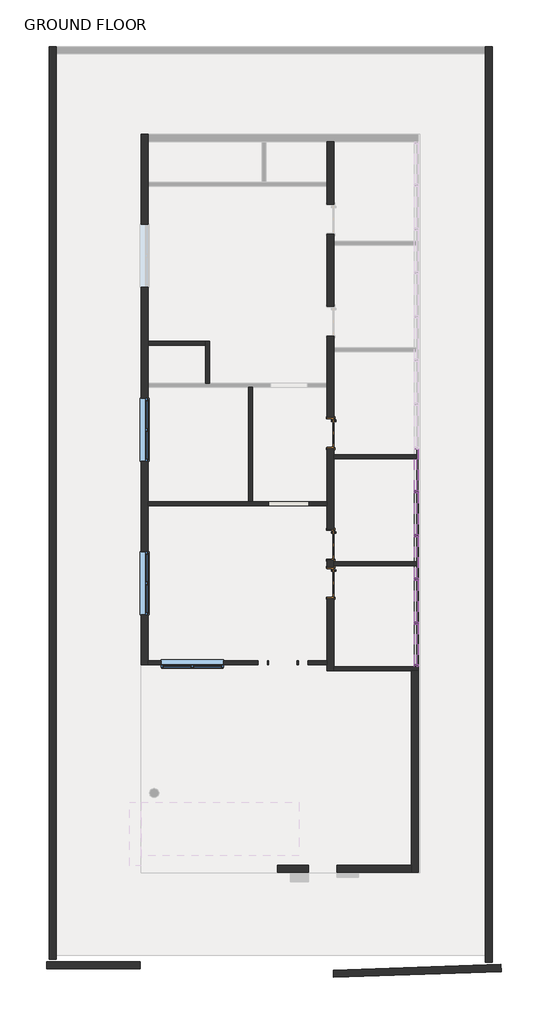
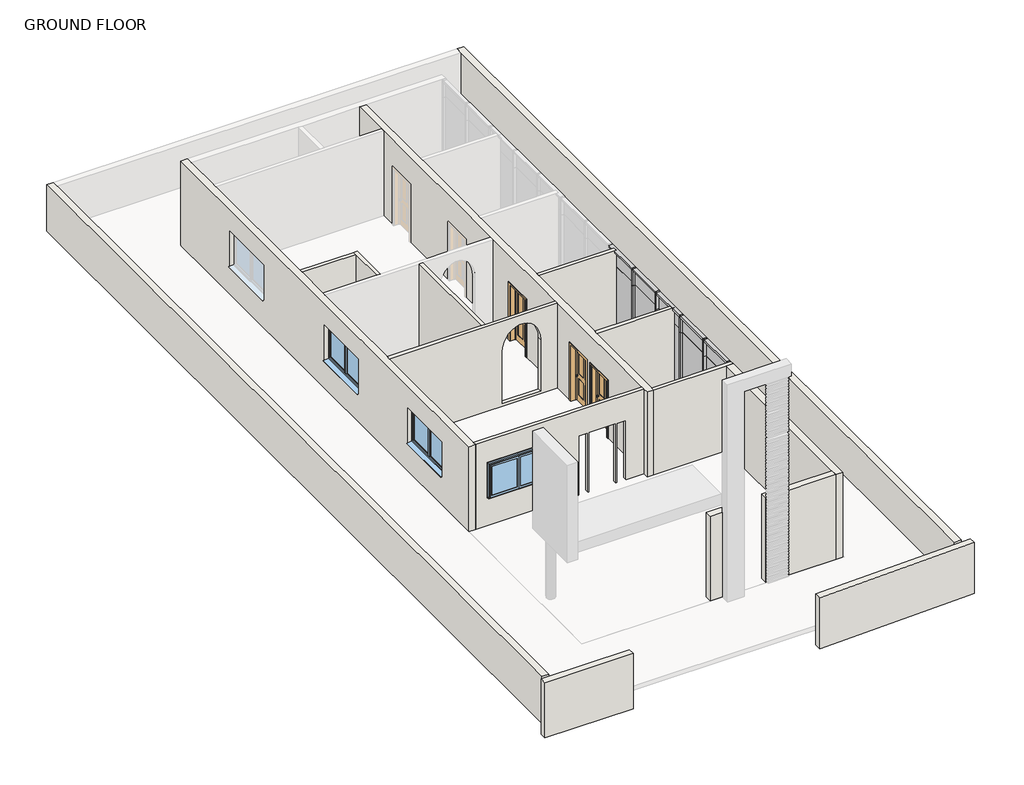
# One storey, part 1 of 2: 19 members, 16 walls, 10 plates, 3 doors, 3 windows.
"""IFC4 building model written with IfcOpenShell, lengths in millimetres."""

from ifc_helpers import new_model, si_unit, point, frame, origin, origin_with_axes, place, context, project, spatial, polyline, ellipse_curve, trimmed, outline, extrude, faceted_brep, transform, mapped, element, save
from ifc_brep_helpers import plane_surface, extruded_surface, advanced_brep
from components import door_8a5afc22, member_fe35c162, member_c919ac1a, member_ee409385, member_47bfaf8a, member_f0fea5a5, member_6e77e263, system_panel_glazed_23a28a9f, system_panel_glazed_17e06366, system_panel_glazed_701ad94b, system_panel_glazed_1ceb456a, w2_0001_w2_7b90d420, w2_0001_w2_6e690f8f

model = new_model("IFC4")

# Units and contexts
model_context = context("Model", 3, world=origin())
ifc_project = project(units=[si_unit("LENGTHUNIT", "METRE", prefix="MILLI")], contexts=[model_context])

# Site, building, storey
site = spatial("IfcSite", under=ifc_project)
building = spatial("IfcBuilding", under=site)
storey = spatial("IfcBuildingStorey", under=building, Name="GROUND FLOOR", Elevation=304.8)

# Doors
placement = place(None, origin())
door_shape = door_8a5afc22(model_context)
element("IfcDoor", 1, ObjectType="Door-Interior-Single-4_Panel-Wood : 36\" x 80\"", at=placement, inside=storey, context=model_context, shape_type="MappedRepresentation", body=[
    mapped(door_shape, transform((7334.4173568, -4256.3073314, 304.8), x_axis=(0.0, -1.0, 0.0), y_axis=(1.0, 0.0, 0.0), z_axis=(0.0, 0.0, 1.0))),
])
element("IfcDoor", 2, ObjectType="Door-Interior-Single-4_Panel-Wood : 36\" x 80\"", at=placement, inside=storey, context=model_context, shape_type="MappedRepresentation", body=[
    mapped(door_shape, transform((7334.4173568, -3037.1073314, 304.8), x_axis=(0.0, -1.0, 0.0), y_axis=(1.0, 0.0, 0.0), z_axis=(0.0, 0.0, 1.0))),
])
element("IfcDoor", 3, ObjectType="Door-Interior-Single-4_Panel-Wood : 36\" x 80\"", at=placement, inside=storey, context=model_context, shape_type="MappedRepresentation", body=[
    mapped(door_shape, transform((7334.4173568, 531.5926686, 304.8), x_axis=(0.0, -1.0, 0.0), y_axis=(1.0, 0.0, 0.0), z_axis=(0.0, 0.0, 1.0))),
])

# Members
member_shape = member_fe35c162(model_context)
element("IfcMember", 4, ObjectType="Rectangular Mullion : 2.5\" x 5\" rectangular", at=placement, inside=storey, context=model_context, shape_type="MappedRepresentation", body=[
    mapped(member_shape, transform((10074.4423568, -5569.6989978, 304.8), x_axis=(0.0, 0.0, -1.0), y_axis=(-1.0, 0.0, 0.0), z_axis=(0.0, 1.0, 0.0))),
])
element("IfcMember", 5, ObjectType="Rectangular Mullion : 2.5\" x 5\" rectangular", at=placement, inside=storey, context=model_context, shape_type="MappedRepresentation", body=[
    mapped(member_shape, transform((10074.4423568, -6872.5073314, 3352.8), x_axis=(0.0, 0.0, 1.0), y_axis=(-1.0, 0.0, 0.0), z_axis=(0.0, -1.0, 0.0))),
])
member_2_shape = member_c919ac1a(model_context)
element("IfcMember", 6, ObjectType="Rectangular Mullion : 2.5\" x 5\" rectangular", at=placement, inside=storey, context=model_context, shape_type="MappedRepresentation", body=[
    mapped(member_2_shape, transform((10074.4423568, -1312.023998, 3352.8), x_axis=(0.0, 0.0, 1.0), y_axis=(-1.0, 0.0, 0.0), z_axis=(0.0, -1.0, 0.0))),
])
element("IfcMember", 7, ObjectType="Rectangular Mullion : 2.5\" x 5\" rectangular", at=placement, inside=storey, context=model_context, shape_type="MappedRepresentation", body=[
    mapped(member_2_shape, transform((10074.4423568, -2710.0823312, 3352.8), x_axis=(0.0, 0.0, 1.0), y_axis=(-1.0, 0.0, 0.0), z_axis=(0.0, -1.0, 0.0))),
])
element("IfcMember", 8, ObjectType="Rectangular Mullion : 2.5\" x 5\" rectangular", at=placement, inside=storey, context=model_context, shape_type="MappedRepresentation", body=[
    mapped(member_2_shape, transform((10074.4423568, -4108.1406645, 3352.8), x_axis=(0.0, 0.0, 1.0), y_axis=(-1.0, 0.0, 0.0), z_axis=(0.0, -1.0, 0.0))),
])
element("IfcMember", 9, ObjectType="Rectangular Mullion : 2.5\" x 5\" rectangular", at=placement, inside=storey, context=model_context, shape_type="MappedRepresentation", body=[
    mapped(member_2_shape, transform((10074.4423568, -5506.1989978, 3352.8), x_axis=(0.0, 0.0, 1.0), y_axis=(-1.0, 0.0, 0.0), z_axis=(0.0, -1.0, 0.0))),
])
element("IfcMember", 10, ObjectType="Rectangular Mullion : 2.5\" x 5\" rectangular", at=placement, inside=storey, context=model_context, shape_type="MappedRepresentation", body=[
    mapped(member_2_shape, transform((10074.4423568, -1375.523998, 304.8), x_axis=(0.0, 0.0, -1.0), y_axis=(-1.0, 0.0, 0.0), z_axis=(0.0, 1.0, 0.0))),
])
element("IfcMember", 11, ObjectType="Rectangular Mullion : 2.5\" x 5\" rectangular", at=placement, inside=storey, context=model_context, shape_type="MappedRepresentation", body=[
    mapped(member_2_shape, transform((10074.4423568, -2773.5823312, 304.8), x_axis=(0.0, 0.0, -1.0), y_axis=(-1.0, 0.0, 0.0), z_axis=(0.0, 1.0, 0.0))),
])
element("IfcMember", 12, ObjectType="Rectangular Mullion : 2.5\" x 5\" rectangular", at=placement, inside=storey, context=model_context, shape_type="MappedRepresentation", body=[
    mapped(member_2_shape, transform((10074.4423568, -4171.6406645, 304.8), x_axis=(0.0, 0.0, -1.0), y_axis=(-1.0, 0.0, 0.0), z_axis=(0.0, 1.0, 0.0))),
])
member_3_shape = member_ee409385(model_context)
element("IfcMember", 13, ObjectType="Rectangular Mullion : 2.5\" x 5\" rectangular", at=placement, inside=storey, context=model_context, shape_type="MappedRepresentation", body=[
    mapped(member_3_shape, transform((10074.4423568, -6936.0073314, 304.8), x_axis=(0.0, -1.0, 0.0), y_axis=(-1.0, 0.0, 0.0), z_axis=(0.0, 0.0, -1.0))),
])
member_4_shape = member_47bfaf8a(model_context)
element("IfcMember", 14, ObjectType="Rectangular Mullion : 2.5\" x 5\" rectangular", at=placement, inside=storey, context=model_context, shape_type="MappedRepresentation", body=[
    mapped(member_4_shape, transform((10074.4423568, -6936.0073314, 2743.2), x_axis=(0.0, -1.0, 0.0), y_axis=(-1.0, 0.0, 0.0), z_axis=(0.0, 0.0, -1.0))),
])
member_5_shape = member_f0fea5a5(model_context)
element("IfcMember", 15, ObjectType="Rectangular Mullion : 2.5\" x 5\" rectangular", at=placement, inside=storey, context=model_context, shape_type="MappedRepresentation", body=[
    mapped(member_5_shape, transform((10074.4423568, -1343.773998, 304.8), x_axis=(0.0, -1.0, 0.0), y_axis=(-1.0, 0.0, 0.0), z_axis=(0.0, 0.0, -1.0))),
])
element("IfcMember", 16, ObjectType="Rectangular Mullion : 2.5\" x 5\" rectangular", at=placement, inside=storey, context=model_context, shape_type="MappedRepresentation", body=[
    mapped(member_5_shape, transform((10074.4423568, -2741.8323312, 304.8), x_axis=(0.0, -1.0, 0.0), y_axis=(-1.0, 0.0, 0.0), z_axis=(0.0, 0.0, -1.0))),
])
element("IfcMember", 17, ObjectType="Rectangular Mullion : 2.5\" x 5\" rectangular", at=placement, inside=storey, context=model_context, shape_type="MappedRepresentation", body=[
    mapped(member_5_shape, transform((10074.4423568, -4139.8906645, 304.8), x_axis=(0.0, -1.0, 0.0), y_axis=(-1.0, 0.0, 0.0), z_axis=(0.0, 0.0, -1.0))),
])
element("IfcMember", 18, ObjectType="Rectangular Mullion : 2.5\" x 5\" rectangular", at=placement, inside=storey, context=model_context, shape_type="MappedRepresentation", body=[
    mapped(member_5_shape, transform((10074.4423568, -5537.9489978, 304.8), x_axis=(0.0, -1.0, 0.0), y_axis=(-1.0, 0.0, 0.0), z_axis=(0.0, 0.0, -1.0))),
])
member_6_shape = member_6e77e263(model_context)
element("IfcMember", 19, ObjectType="Rectangular Mullion : 2.5\" x 5\" rectangular", at=placement, inside=storey, context=model_context, shape_type="MappedRepresentation", body=[
    mapped(member_6_shape, transform((10074.4423568, -1343.773998, 2743.2), x_axis=(0.0, -1.0, 0.0), y_axis=(-1.0, 0.0, 0.0), z_axis=(0.0, 0.0, -1.0))),
])
element("IfcMember", 20, ObjectType="Rectangular Mullion : 2.5\" x 5\" rectangular", at=placement, inside=storey, context=model_context, shape_type="MappedRepresentation", body=[
    mapped(member_6_shape, transform((10074.4423568, -2741.8323312, 2743.2), x_axis=(0.0, -1.0, 0.0), y_axis=(-1.0, 0.0, 0.0), z_axis=(0.0, 0.0, -1.0))),
])
element("IfcMember", 21, ObjectType="Rectangular Mullion : 2.5\" x 5\" rectangular", at=placement, inside=storey, context=model_context, shape_type="MappedRepresentation", body=[
    mapped(member_6_shape, transform((10074.4423568, -4139.8906645, 2743.2), x_axis=(0.0, -1.0, 0.0), y_axis=(-1.0, 0.0, 0.0), z_axis=(0.0, 0.0, -1.0))),
])
element("IfcMember", 22, ObjectType="Rectangular Mullion : 2.5\" x 5\" rectangular", at=placement, inside=storey, context=model_context, shape_type="MappedRepresentation", body=[
    mapped(member_6_shape, transform((10074.4423568, -5537.9489978, 2743.2), x_axis=(0.0, -1.0, 0.0), y_axis=(-1.0, 0.0, 0.0), z_axis=(0.0, 0.0, -1.0))),
])

# Plates
system_panel_glazed_shape = system_panel_glazed_23a28a9f(model_context)
element("IfcPlate", 23, ObjectType="System Panel : Glazed", at=placement, inside=storey, context=model_context, shape_type="MappedRepresentation", body=[
    mapped(system_panel_glazed_shape, transform((10074.4423568, -6221.1031646, 368.3), x_axis=(0.0, -1.0, 0.0), y_axis=(1.0, 0.0, 0.0), z_axis=(0.0, 0.0, 1.0))),
])
system_panel_glazed_2_shape = system_panel_glazed_17e06366(model_context)
element("IfcPlate", 24, ObjectType="System Panel : Glazed", at=placement, inside=storey, context=model_context, shape_type="MappedRepresentation", body=[
    mapped(system_panel_glazed_2_shape, transform((10074.4423568, -6221.1031646, 2743.2), x_axis=(0.0, -1.0, 0.0), y_axis=(1.0, 0.0, 0.0), z_axis=(0.0, 0.0, 1.0))),
])
system_panel_glazed_3_shape = system_panel_glazed_701ad94b(model_context)
element("IfcPlate", 25, ObjectType="System Panel : Glazed", at=placement, inside=storey, context=model_context, shape_type="MappedRepresentation", body=[
    mapped(system_panel_glazed_3_shape, transform((10074.4423568, -644.7448313, 368.3), x_axis=(0.0, -1.0, 0.0), y_axis=(1.0, 0.0, 0.0), z_axis=(0.0, 0.0, 1.0))),
])
element("IfcPlate", 26, ObjectType="System Panel : Glazed", at=placement, inside=storey, context=model_context, shape_type="MappedRepresentation", body=[
    mapped(system_panel_glazed_3_shape, transform((10074.4423568, -2042.8031646, 368.3), x_axis=(0.0, -1.0, 0.0), y_axis=(1.0, 0.0, 0.0), z_axis=(0.0, 0.0, 1.0))),
])
element("IfcPlate", 27, ObjectType="System Panel : Glazed", at=placement, inside=storey, context=model_context, shape_type="MappedRepresentation", body=[
    mapped(system_panel_glazed_3_shape, transform((10074.4423568, -3440.8614979, 368.3), x_axis=(0.0, -1.0, 0.0), y_axis=(1.0, 0.0, 0.0), z_axis=(0.0, 0.0, 1.0))),
])
element("IfcPlate", 28, ObjectType="System Panel : Glazed", at=placement, inside=storey, context=model_context, shape_type="MappedRepresentation", body=[
    mapped(system_panel_glazed_3_shape, transform((10074.4423568, -4838.9198312, 368.3), x_axis=(0.0, -1.0, 0.0), y_axis=(1.0, 0.0, 0.0), z_axis=(0.0, 0.0, 1.0))),
])
system_panel_glazed_4_shape = system_panel_glazed_1ceb456a(model_context)
element("IfcPlate", 29, ObjectType="System Panel : Glazed", at=placement, inside=storey, context=model_context, shape_type="MappedRepresentation", body=[
    mapped(system_panel_glazed_4_shape, transform((10074.4423568, -644.7448313, 2743.2), x_axis=(0.0, -1.0, 0.0), y_axis=(1.0, 0.0, 0.0), z_axis=(0.0, 0.0, 1.0))),
])
element("IfcPlate", 30, ObjectType="System Panel : Glazed", at=placement, inside=storey, context=model_context, shape_type="MappedRepresentation", body=[
    mapped(system_panel_glazed_4_shape, transform((10074.4423568, -2042.8031646, 2743.2), x_axis=(0.0, -1.0, 0.0), y_axis=(1.0, 0.0, 0.0), z_axis=(0.0, 0.0, 1.0))),
])
element("IfcPlate", 31, ObjectType="System Panel : Glazed", at=placement, inside=storey, context=model_context, shape_type="MappedRepresentation", body=[
    mapped(system_panel_glazed_4_shape, transform((10074.4423568, -3440.8614979, 2743.2), x_axis=(0.0, -1.0, 0.0), y_axis=(1.0, 0.0, 0.0), z_axis=(0.0, 0.0, 1.0))),
])
element("IfcPlate", 32, ObjectType="System Panel : Glazed", at=placement, inside=storey, context=model_context, shape_type="MappedRepresentation", body=[
    mapped(system_panel_glazed_4_shape, transform((10074.4423568, -4838.9198312, 2743.2), x_axis=(0.0, -1.0, 0.0), y_axis=(1.0, 0.0, 0.0), z_axis=(0.0, 0.0, 1.0))),
])

# Walls
element("IfcWall", 33, ObjectType="INNER WALL 5\"", at=placement, inside=storey, context=model_context, shape_type="SweptSolid", body=[
    extrude(outline(polyline([(7445.5423568, -166.9073314), (10074.4423568, -166.9073314), (10074.4423568, -293.9073314), (7445.5423568, -293.9073314), (7445.5423568, -166.9073314)])), frame((0.0, 0.0, 304.8), z_axis=(0.0, 0.0, 1.0), x_axis=(1.0, 0.0, 0.0)), (0.0, 0.0, 1.0), 3048.0),
])
element("IfcWall", 34, ObjectType="INNER WALL 5\"", at=placement, inside=storey, context=model_context, shape_type="SweptSolid", body=[
    extrude(outline(polyline([(7445.5423568, -3583.2073314), (10074.4423568, -3583.2073314), (10074.4423568, -3710.2073314), (7445.5423568, -3710.2073314), (7445.5423568, -3583.2073314)])), frame((0.0, 0.0, 304.8), z_axis=(0.0, 0.0, 1.0), x_axis=(1.0, 0.0, 0.0)), (0.0, 0.0, 1.0), 3048.0),
])
element("IfcWall", 35, ObjectType="INNER WALL 5\"", at=placement, inside=storey, context=model_context, shape_type="Brep", body=[
    faceted_brep([(7445.5423568, -7063.0073314, 304.8), (9909.3423568, -7063.0073314, 304.8), (10137.9423568, -7063.0073314, 304.8), (10137.9423568, -7063.0073314, 3352.8), (9909.3423568, -7063.0073314, 3352.8), (7445.5423568, -7063.0073314, 3352.8), (7445.5423568, -6936.0073314, 304.8), (7445.5423568, -6936.0073314, 3352.8), (10137.9423568, -6936.0073314, 3352.8), (10137.9423568, -6936.0073314, 304.8)], [[[0, 1, 2, 3, 4, 5]], [[6, 7, 8, 9]], [[2, 1, 0, 6, 9]], [[5, 4, 3, 8, 7]], [[0, 5, 7, 6]], [[3, 2, 9, 8]]]),
])
element("IfcWall", 36, ObjectType="INNER WALL 5\"", at=placement, inside=storey, context=model_context, shape_type="SweptSolid", body=[
    extrude(outline(polyline([(1501.9423568, 3465.2926686), (3330.7423568, 3465.2926686), (3330.7423568, 3338.2926686), (1501.9423568, 3338.2926686), (1501.9423568, 3465.2926686)])), frame((0.0, 0.0, 304.8), z_axis=(0.0, 0.0, 1.0), x_axis=(1.0, 0.0, 0.0)), (0.0, 0.0, 1.0), 3048.0),
])
element("IfcWall", 37, ObjectType="INNER WALL 5\"", at=placement, inside=storey, context=model_context, shape_type="AdvancedBrep", body=[
    advanced_brep(
    [(7216.9423568, -1665.5073314, 304.8), (4829.3423568, -1665.5073314, 304.8), (4702.3423568, -1665.5073314, 304.8), (1501.9423568, -1665.5073314, 304.8), (1501.9423568, -1665.5073314, 3352.8), (4702.3423568, -1665.5073314, 3352.8), (4829.3423568, -1665.5073314, 3352.8), (7216.9423568, -1665.5073314, 3352.8), (5348.459588, -1665.5073314, 397.3174472), (6643.859588, -1665.5073314, 397.3174472), (6643.859588, -1665.5073314, 2251.5174472), (5348.459588, -1665.5073314, 2251.5174472), (7216.9423568, -1792.5073314, 304.8), (7216.9423568, -1792.5073314, 3352.8), (1501.9423568, -1792.5073314, 3352.8), (1501.9423568, -1792.5073314, 304.8), (5348.459588, -1792.5073314, 397.3174472), (5348.459588, -1792.5073314, 2251.5174472), (6643.859588, -1792.5073314, 2251.5174472), (6643.859588, -1792.5073314, 397.3174472)],
    [
        (0, 1),
        (1, 2),
        (2, 3),
        (3, 4),
        (4, 5),
        (5, 6),
        (6, 7),
        (7, 0),
        (8, 9),
        (9, 10),
        (10, 11, ellipse_curve(frame((5996.159588, -1665.5073314, 2251.5174472), z_axis=(0.0, -1.0, 0.0), x_axis=(0.0, 0.0, -1.0)), 787.4, 647.7)),
        (11, 8),
        (12, 13),
        (13, 14),
        (14, 15),
        (15, 12),
        (16, 17),
        (17, 18, ellipse_curve(frame((5996.159588, -1792.5073314, 2251.5174472), z_axis=(0.0, 1.0, 0.0), x_axis=(0.0, 0.0, -1.0)), 787.4, 647.7)),
        (18, 19),
        (19, 16),
        (3, 15),
        (14, 4),
        (7, 13),
        (12, 0),
        (8, 16),
        (19, 9),
        (18, 10),
        (17, 11),
    ],
    [
        plane_surface(frame((7331.2423568, -1665.5073314, 304.8), z_axis=(0.0, 1.0, 0.0), x_axis=(-1.0, 0.0, 0.0))),
        plane_surface(frame((7331.2423568, -1792.5073314, 304.8), z_axis=(0.0, -1.0, 0.0), x_axis=(1.0, 0.0, 0.0))),
        plane_surface(frame((1501.9423568, -8333.0073314, 304.8), z_axis=(-1.0, 0.0, 0.0), x_axis=(0.0, 1.0, 0.0))),
        plane_surface(frame((7216.9423568, 9954.9926686, 304.8), z_axis=(1.0, 0.0, 0.0), x_axis=(0.0, -1.0, 0.0))),
        plane_surface(frame((7331.2423568, -1665.5073314, 304.8), z_axis=(0.0, 0.0, -1.0), x_axis=(0.0, -1.0, 0.0))),
        plane_surface(frame((1387.6423568, -1665.5073314, 3352.8), z_axis=(0.0, 0.0, 1.0), x_axis=(0.0, -1.0, 0.0))),
        plane_surface(frame((5348.459588, -1665.5073314, 397.3174472), z_axis=(0.0, 0.0, 1.0), x_axis=(0.0, -1.0, 0.0))),
        plane_surface(frame((6643.859588, -1665.5073314, 397.3174472), z_axis=(-1.0, 0.0, 0.0), x_axis=(0.0, -1.0, 0.0))),
        extruded_surface(trimmed(ellipse_curve(frame((5996.159588, -1856.0073314, 2251.5174472), z_axis=(0.0, -1.0, 0.0), x_axis=(-1.0, 0.0, 0.0)), 647.7, 787.4), [point((6643.859588, -1856.0073314, 2251.5174472))], [point((5348.459588, -1856.0073314, 2251.5174472))], True, "CARTESIAN"), (0.0, 127.0, 0.0), 127.0),
        plane_surface(frame((5348.459588, -1665.5073314, 2251.5174472), z_axis=(1.0, 0.0, 0.0), x_axis=(0.0, -1.0, 0.0))),
    ],
    [
        (0, [[1, 2, 3, 4, 5, 6, 7, 8], [9, 10, 11, 12]]),
        (1, [[13, 14, 15, 16], [17, 18, 19, 20]]),
        (2, [[-4, 21, -15, 22]]),
        (3, [[-8, 23, -13, 24]]),
        (4, [[-3, -2, -1, -24, -16, -21]]),
        (5, [[-7, -6, -5, -22, -14, -23]]),
        (6, [[-9, 25, -20, 26]]),
        (7, [[-10, -26, -19, 27]]),
        (8, [[-11, -27, -18, 28]]),
        (9, [[-12, -28, -17, -25]]),
    ],
),
])
element("IfcWall", 38, ObjectType="INNER WALL 5\"", at=placement, inside=storey, context=model_context, shape_type="SweptSolid", body=[
    extrude(outline(polyline([(304.8, 1501.9423568), (304.8, 5007.1423568), (2438.4, 5007.1423568), (2438.4, 5311.9423568), (304.8, 5311.9423568), (304.8, 5350.0423568), (2438.4, 5350.0423568), (2438.4, 6264.4423568), (304.8, 6264.4423568), (304.8, 6302.5423568), (2438.4, 6302.5423568), (2438.4, 6607.3423568), (304.8, 6607.3423568), (304.8, 7216.9423568), (3352.8, 7216.9423568), (3352.8, 1501.9423568), (304.8, 1501.9423568)]), holes=[polyline([(1304.8, 3916.6423568), (1304.8, 1906.6423568), (2564.8, 1906.6423568), (2564.8, 3916.6423568), (1304.8, 3916.6423568)])]), frame((0.0, -6872.5073314, 0.0), z_axis=(0.0, 1.0, 0.0), x_axis=(0.0, 0.0, 1.0)), (0.0, 0.0, 1.0), 127.0),
])
element("IfcWall", 39, ObjectType="INNER WALL 5\"", at=placement, inside=storey, context=model_context, shape_type="SweptSolid", body=[
    extrude(outline(polyline([(4702.3423568, -1665.5073314), (4702.3423568, 1992.0926686), (4829.3423568, 1992.0926686), (4829.3423568, -1665.5073314), (4702.3423568, -1665.5073314)])), frame((0.0, 0.0, 304.8), z_axis=(0.0, 0.0, 1.0), x_axis=(1.0, 0.0, 0.0)), (0.0, 0.0, 1.0), 3048.0),
])
element("IfcWall", 40, ObjectType="INNER WALL 5\"", at=placement, inside=storey, context=model_context, shape_type="Brep", body=[
    faceted_brep([(3330.7423568, 3465.2926686, 304.8), (3330.7423568, 3338.2926686, 304.8), (3330.7423568, 2119.0926686, 304.8), (3330.7423568, 2119.0926686, 3352.8), (3330.7423568, 3338.2926686, 3352.8), (3330.7423568, 3465.2926686, 3352.8), (3457.7423568, 3465.2926686, 304.8), (3457.7423568, 3465.2926686, 3352.8), (3457.7423568, 2119.0926686, 3352.8), (3457.7423568, 2119.0926686, 304.8)], [[[0, 1, 2, 3, 4, 5]], [[6, 7, 8, 9]], [[2, 1, 0, 6, 9]], [[5, 4, 3, 8, 7]], [[3, 2, 9, 8]], [[0, 5, 7, 6]]]),
])
element("IfcWall", 41, ObjectType="OUTER WALL 9\"", at=placement, inside=storey, context=model_context, shape_type="Brep", body=[
    faceted_brep([(1501.9423568, -6872.5073314, 304.8), (1501.9423568, -6745.5073314, 304.8), (1501.9423568, -1792.5073314, 304.8), (1501.9423568, -1665.5073314, 304.8), (1501.9423568, 1992.0926686, 304.8), (1501.9423568, 2119.0926686, 304.8), (1501.9423568, 3338.2926686, 304.8), (1501.9423568, 3465.2926686, 304.8), (1501.9423568, 8418.2926686, 304.8), (1501.9423568, 8545.2926686, 304.8), (1501.9423568, 9840.6926686, 304.8), (1501.9423568, 10069.2926686, 304.8), (1501.9423568, 10069.2926686, 3352.8), (1501.9423568, 9840.6926686, 3352.8), (1501.9423568, 8545.2926686, 3352.8), (1501.9423568, 8418.2926686, 3352.8), (1501.9423568, 3465.2926686, 3352.8), (1501.9423568, 3338.2926686, 3352.8), (1501.9423568, 2119.0926686, 3352.8), (1501.9423568, 1992.0926686, 3352.8), (1501.9423568, -1665.5073314, 3352.8), (1501.9423568, -1792.5073314, 3352.8), (1501.9423568, -6745.5073314, 3352.8), (1501.9423568, -6872.5073314, 3352.8), (1501.9423568, -5274.0073314, 1304.8), (1501.9423568, -5274.0073314, 2564.8), (1501.9423568, -3264.0073314, 2564.8), (1501.9423568, -3264.0073314, 1304.8), (1501.9423568, -371.8073314, 1304.8), (1501.9423568, -371.8073314, 2564.8), (1501.9423568, 1638.1926686, 2564.8), (1501.9423568, 1638.1926686, 1304.8), (1501.9423568, 5190.7926686, 1304.8), (1501.9423568, 5190.7926686, 2564.8), (1501.9423568, 7200.7926686, 2564.8), (1501.9423568, 7200.7926686, 1304.8), (1273.3423568, -6872.5073314, 304.8), (1273.3423568, -6872.5073314, 3352.8), (1273.3423568, 10069.2926686, 3352.8), (1273.3423568, 10069.2926686, 304.8), (1273.3423568, -5274.0073314, 1304.8), (1273.3423568, -3264.0073314, 1304.8), (1273.3423568, -3264.0073314, 2564.8), (1273.3423568, -5274.0073314, 2564.8), (1273.3423568, -371.8073314, 1304.8), (1273.3423568, 1638.1926686, 1304.8), (1273.3423568, 1638.1926686, 2564.8), (1273.3423568, -371.8073314, 2564.8), (1273.3423568, 5190.7926686, 1304.8), (1273.3423568, 7200.7926686, 1304.8), (1273.3423568, 7200.7926686, 2564.8), (1273.3423568, 5190.7926686, 2564.8)], [[[0, 1, 2, 3, 4, 5, 6, 7, 8, 9, 10, 11, 12, 13, 14, 15, 16, 17, 18, 19, 20, 21, 22, 23], [24, 25, 26, 27], [28, 29, 30, 31], [32, 33, 34, 35]], [[36, 37, 38, 39], [40, 41, 42, 43], [44, 45, 46, 47], [48, 49, 50, 51]], [[11, 10, 9, 8, 7, 6, 5, 4, 3, 2, 1, 0, 36, 39]], [[23, 22, 21, 20, 19, 18, 17, 16, 15, 14, 13, 12, 38, 37]], [[12, 11, 39, 38]], [[0, 23, 37, 36]], [[25, 24, 40, 43]], [[26, 25, 43, 42]], [[27, 26, 42, 41]], [[24, 27, 41, 40]], [[29, 28, 44, 47]], [[30, 29, 47, 46]], [[31, 30, 46, 45]], [[28, 31, 45, 44]], [[33, 32, 48, 51]], [[34, 33, 51, 50]], [[35, 34, 50, 49]], [[32, 35, 49, 48]]]),
])
element("IfcWall", 42, ObjectType="OUTER WALL 9\"", at=placement, inside=storey, context=model_context, shape_type="Brep", body=[
    faceted_brep([(7216.9423568, -7063.0073314, 3352.8), (7216.9423568, -6872.5073314, 3352.8), (7216.9423568, -6745.5073314, 3352.8), (7216.9423568, -1792.5073314, 3352.8), (7216.9423568, -1665.5073314, 3352.8), (7216.9423568, 1992.0926686, 3352.8), (7216.9423568, 2119.0926686, 3352.8), (7216.9423568, 8418.2926686, 3352.8), (7216.9423568, 8545.2926686, 3352.8), (7216.9423568, 9840.6926686, 3352.8), (7216.9423568, 9840.6926686, 304.8), (7216.9423568, 8545.2926686, 304.8), (7216.9423568, 8418.2926686, 304.8), (7216.9423568, 7846.7926686, 304.8), (7216.9423568, 7846.7926686, 2362.2), (7216.9423568, 6881.5926686, 2362.2), (7216.9423568, 6881.5926686, 304.8), (7216.9423568, 4582.8926686, 304.8), (7216.9423568, 4582.8926686, 2362.2), (7216.9423568, 3617.6926686, 2362.2), (7216.9423568, 3617.6926686, 304.8), (7216.9423568, 2119.0926686, 304.8), (7216.9423568, 1992.0926686, 304.8), (7216.9423568, 1014.1926686, 304.8), (7216.9423568, 1014.1926686, 2362.2), (7216.9423568, 48.9926686, 2362.2), (7216.9423568, 48.9926686, 304.8), (7216.9423568, -1665.5073314, 304.8), (7216.9423568, -1792.5073314, 304.8), (7216.9423568, -2554.5073314, 304.8), (7216.9423568, -2554.5073314, 2362.2), (7216.9423568, -3519.7073314, 2362.2), (7216.9423568, -3519.7073314, 304.8), (7216.9423568, -3773.7073314, 304.8), (7216.9423568, -3773.7073314, 2362.2), (7216.9423568, -4738.9073314, 2362.2), (7216.9423568, -4738.9073314, 304.8), (7216.9423568, -6745.5073314, 304.8), (7216.9423568, -6872.5073314, 304.8), (7216.9423568, -7063.0073314, 304.8), (7445.5423568, 9840.6926686, 3352.8), (7445.5423568, 6665.6926686, 3352.8), (7445.5423568, 6538.6926686, 3352.8), (7445.5423568, 3249.3926686, 3352.8), (7445.5423568, 3122.3926686, 3352.8), (7445.5423568, -166.9073314, 3352.8), (7445.5423568, -293.9073314, 3352.8), (7445.5423568, -3583.2073314, 3352.8), (7445.5423568, -3710.2073314, 3352.8), (7445.5423568, -6936.0073314, 3352.8), (7445.5423568, -7063.0073314, 3352.8), (7445.5423568, -7063.0073314, 304.8), (7445.5423568, -6936.0073314, 304.8), (7445.5423568, -4738.9073314, 304.8), (7445.5423568, -4738.9073314, 2362.2), (7445.5423568, -3773.7073314, 2362.2), (7445.5423568, -3773.7073314, 304.8), (7445.5423568, -3710.2073314, 304.8), (7445.5423568, -3583.2073314, 304.8), (7445.5423568, -3519.7073314, 304.8), (7445.5423568, -3519.7073314, 2362.2), (7445.5423568, -2554.5073314, 2362.2), (7445.5423568, -2554.5073314, 304.8), (7445.5423568, -293.9073314, 304.8), (7445.5423568, -166.9073314, 304.8), (7445.5423568, 48.9926686, 304.8), (7445.5423568, 48.9926686, 2362.2), (7445.5423568, 1014.1926686, 2362.2), (7445.5423568, 1014.1926686, 304.8), (7445.5423568, 3122.3926686, 304.8), (7445.5423568, 3249.3926686, 304.8), (7445.5423568, 3617.6926686, 304.8), (7445.5423568, 3617.6926686, 2362.2), (7445.5423568, 4582.8926686, 2362.2), (7445.5423568, 4582.8926686, 304.8), (7445.5423568, 6538.6926686, 304.8), (7445.5423568, 6665.6926686, 304.8), (7445.5423568, 6881.5926686, 304.8), (7445.5423568, 6881.5926686, 2362.2), (7445.5423568, 7846.7926686, 2362.2), (7445.5423568, 7846.7926686, 304.8), (7445.5423568, 9840.6926686, 304.8)], [[[0, 1, 2, 3, 4, 5, 6, 7, 8, 9, 10, 11, 12, 13, 14, 15, 16, 17, 18, 19, 20, 21, 22, 23, 24, 25, 26, 27, 28, 29, 30, 31, 32, 33, 34, 35, 36, 37, 38, 39]], [[40, 41, 42, 43, 44, 45, 46, 47, 48, 49, 50, 51, 52, 53, 54, 55, 56, 57, 58, 59, 60, 61, 62, 63, 64, 65, 66, 67, 68, 69, 70, 71, 72, 73, 74, 75, 76, 77, 78, 79, 80, 81]], [[10, 81, 80, 13, 12, 11]], [[51, 39, 38, 37, 36, 53, 52]], [[56, 33, 32, 59, 58, 57]], [[62, 29, 28, 27, 26, 65, 64, 63]], [[68, 23, 22, 21, 20, 71, 70, 69]], [[74, 17, 16, 77, 76, 75]], [[9, 8, 7, 6, 5, 4, 3, 2, 1, 0, 50, 49, 48, 47, 46, 45, 44, 43, 42, 41, 40]], [[10, 9, 40, 81]], [[0, 39, 51, 50]], [[35, 54, 53, 36]], [[54, 35, 34, 55]], [[55, 34, 33, 56]], [[31, 60, 59, 32]], [[60, 31, 30, 61]], [[61, 30, 29, 62]], [[25, 66, 65, 26]], [[66, 25, 24, 67]], [[67, 24, 23, 68]], [[19, 72, 71, 20]], [[72, 19, 18, 73]], [[73, 18, 17, 74]], [[15, 78, 77, 16]], [[78, 15, 14, 79]], [[79, 14, 13, 80]]]),
])
element("IfcWall", 43, ObjectType="OUTER WALL 9\"", at=placement, inside=storey, context=model_context, shape_type="Brep", body=[
    faceted_brep([(9909.3423568, -7063.0073314, 304.8), (9909.3423568, -13273.3073314, 304.8), (9909.3423568, -13501.9073314, 304.8), (9909.3423568, -13501.9073314, 3352.8), (9909.3423568, -13273.3073314, 3352.8), (9909.3423568, -7063.0073314, 3352.8), (10137.9423568, -7063.0073314, 304.8), (10137.9423568, -7063.0073314, 3352.8), (10137.9423568, -13501.9073314, 3352.8), (10137.9423568, -13501.9073314, 304.8)], [[[0, 1, 2, 3, 4, 5]], [[6, 7, 8, 9]], [[2, 1, 0, 6, 9]], [[5, 4, 3, 8, 7]], [[0, 5, 7, 6]], [[3, 2, 9, 8]]]),
])
element("IfcWall", 44, ObjectType="OUTER WALL 9\"", at=placement, inside=storey, context=model_context, shape_type="SweptSolid", body=[
    extrude(outline(polyline([(5642.1423568, -13501.9073314), (5642.1423568, -13273.3073314), (6619.47371, -13273.3073314), (6619.47371, -13501.9073314), (5642.1423568, -13501.9073314)])), frame((0.0, 0.0, 304.8), z_axis=(0.0, 0.0, 1.0), x_axis=(1.0, 0.0, 0.0)), (0.0, 0.0, 1.0), 3048.0),
    extrude(outline(polyline([(9909.3423568, -13273.3073314), (9909.3423568, -13501.9073314), (7533.87371, -13501.9073314), (7533.87371, -13273.3073314), (9909.3423568, -13273.3073314)])), frame((0.0, 0.0, 304.8), z_axis=(0.0, 0.0, 1.0), x_axis=(1.0, 0.0, 0.0)), (0.0, 0.0, 1.0), 3048.0),
])
element("IfcWall", 45, ObjectType="OUTER WALL 9\"", at=placement, inside=storey, context=model_context, shape_type="Brep", body=[
    faceted_brep([(-1667.1997778, 12877.9739596, 152.4), (-1667.1997778, -16268.5260404, 152.4), (-1667.1997778, -16268.5260404, 1828.8), (-1667.1997778, 12877.9739596, 1828.8), (-1438.5997778, 12877.9739596, 152.4), (-1438.5997778, 12877.9739596, 1828.8), (-1438.5997778, 12649.3739596, 1828.8), (-1438.5997778, -16268.5260404, 1828.8), (-1438.5997778, -16268.5260404, 152.4)], [[[0, 1, 2, 3]], [[4, 5, 6, 7, 8]], [[1, 0, 4, 8]], [[2, 1, 8, 7]], [[3, 2, 7, 6, 5]], [[0, 3, 5, 4]]]),
])
element("IfcWall", 46, ObjectType="OUTER WALL 9\"", at=placement, inside=storey, context=model_context, shape_type="Brep", body=[
    faceted_brep([(12506.0002222, -16370.1260404, 0.0), (12506.0002222, 12877.9739596, 0.0), (12506.0002222, 12877.9739596, 1828.8), (12506.0002222, -16370.1260404, 1828.8), (12277.4002222, -16370.1260404, 0.0), (12277.4002222, -16370.1260404, 1828.8), (12277.4002222, 12649.3739596, 1828.8), (12277.4002222, 12877.9739596, 1828.8), (12277.4002222, 12877.9739596, 0.0), (12277.4002222, 12649.3739596, 0.0)], [[[0, 1, 2, 3]], [[4, 5, 6, 7, 8, 9]], [[1, 0, 4, 9, 8]], [[3, 2, 7, 6, 5]], [[0, 3, 5, 4]], [[2, 1, 8, 7]]]),
])
element("IfcWall", 47, ObjectType="OUTER WALL 9\"", at=placement, inside=storey, context=model_context, shape_type="SweptSolid", body=[
    extrude(outline(polyline([(-1749.82629, -16358.220363), (1247.37371, -16358.220363), (1247.37371, -16586.820363), (-1749.82629, -16586.820363), (-1749.82629, -16358.220363)])), frame((0.0, 0.0, -159.3403515), z_axis=(0.0, 0.0, 1.0), x_axis=(1.0, 0.0, 0.0)), (0.0, 0.0, 1.0), 1988.1403515),
])
element("IfcWall", 48, ObjectType="OUTER WALL 9\"", at=placement, inside=storey, context=model_context, shape_type="SweptSolid", body=[
    extrude(outline(polyline([(7419.57371, -16628.286153), (12775.7873225, -16441.2430521), (12783.7653474, -16669.7037951), (7427.551735, -16856.746896), (7419.57371, -16628.286153)])), origin_with_axes(), (0.0, 0.0, 1.0), 1828.8),
])

# Windows
w2_0001_w2_shape = w2_0001_w2_7b90d420(model_context)
element("IfcWindow", 49, ObjectType="w2.0001 : w2", at=placement, inside=storey, context=model_context, shape_type="MappedRepresentation", body=[
    mapped(w2_0001_w2_shape, transform((1387.6423568, -4269.0073314, 304.8), x_axis=(0.0, 1.0, 0.0), y_axis=(-1.0, 0.0, 0.0), z_axis=(0.0, 0.0, 1.0))),
])
element("IfcWindow", 50, ObjectType="w2.0001 : w2", at=placement, inside=storey, context=model_context, shape_type="MappedRepresentation", body=[
    mapped(w2_0001_w2_shape, transform((1387.6423568, 633.1926686, 304.8), x_axis=(0.0, 1.0, 0.0), y_axis=(-1.0, 0.0, 0.0), z_axis=(0.0, 0.0, 1.0))),
])
w2_0001_w2_2_shape = w2_0001_w2_6e690f8f(model_context)
element("IfcWindow", 51, ObjectType="w2.0001 : w2", at=placement, inside=storey, context=model_context, shape_type="MappedRepresentation", body=[
    mapped(w2_0001_w2_2_shape, transform((2911.6423568, -6809.0073314, 304.8), x_axis=(-1.0, 0.0, 0.0), y_axis=(0.0, -1.0, 0.0), z_axis=(0.0, 0.0, 1.0))),
])

save(model, "model.ifc")

# Revit data of these elements
# Type "Door-Interior-Single-4_Panel-Wood : 36\" x 80\""
#   Type Mark = "9"
#   Assembly Code = "C1020300"
#   Analytic Construction = "Wooden"
#   Top Rail = 0' - 4 11/16"
#   Thickness = 0' - 1 3/8"
#   Thermal Resistance (R) = 2.5876 (h·ft²·°F)/BTU
#   Swing Angle [instance default] = 90.00°
#   Stiles = 0' - 4 3/4"
#   Rough Width = 3' - 2"
#   Rough Height = 6' - 9"
#   Mullion = 0' - 4 1/2"
#   Lock Rail = 0' - 7 1/2"
#   Height = 6' - 8"
#   Width = 3' - 0"
#   Heat Transfer Coefficient (U) = 0.3865 BTU/(h·ft²·°F)
#   Bottom Rail = 0' - 9 1/8"
#   Trim Material = Cherry
#   Panel Material = Cherry
#   Frame Material = Cherry
#   Door Handle Material = Aluminum
#   Visual Light Transmittance = 0
#   Solar Heat Gain Coefficient = 0
#   Wall Closure = (empty or 0)
#   Function = (empty or 0)
# Type "Rectangular Mullion : 2.5\" x 5\" rectangular"
#   built-in parameter 1007304 = 0.416667 (stored number, unit not read)
#   built-in parameter 1007301 = 0.104167 (stored number, unit not read)
#   built-in parameter 1007300 = 0.104167 (stored number, unit not read)
# Type "System Panel : Glazed"
#   Construction Type Id = "GSP4R"
#   Analytic Construction = "1/8 in Pilkington single glazing"
#   Visual Light Transmittance = 0.9
#   Solar Heat Gain Coefficient = 0.86
#   Heat Transfer Coefficient (U) = 1.18115 BTU/(h·ft²·°F)
#   Define Thermal Properties by = 1
# Type "INNER WALL 5\""
#   Assembly Code = "B2010"
#   Layers, outside or top first: 0' - 5" "CREAM BEIGE COLOUR" (function 1)
# Type "OUTER WALL 9\""
#   Assembly Code = "B2010"
#   Layers, outside or top first: 0' - 9" "CREAM BEIGE COLOUR" (function 1)
# Type "w2.0001 : w2"
#   Type Mark = "19"
#   Operation = "DoublePanelVertical"
#   Keynote = "16.05.01"
#   Analytic Construction = "<None>"
#   Rough Width = 6' - 7.13386"
#   Rough Height = 4' - 1.6063"
#   Rahmentiefe = 0' - 2.3622"
#   Rahmenhöhe unten = 0' - 3.14961"
#   Rahmehöhe oben = 0' - 3.14961"
#   Rahmenbreite = 0' - 2.3622"
#   Height = 4' - 1.6063"
#   Flügeltiefe = 0' - 2.3622"
#   Flügelbreite = 0' - 2.3622"
#   Einbautiefe (von außen) [instance default] = 0' - 5.51181"
#   Width = 6' - 7.13386"
#   Kippflügel [instance default] = yes
#   Drehflügel im Grundriß darstellen [instance default] = no
#   Drehflügel [instance default] = yes
#   Define Thermal Properties by = 1
#   Rahmen [instance default] = none
#   Glas [instance default] = none
#   Flügel [instance default] = none
#   Fensterbank aussen [instance default] = none
#   Fensterbank innen [instance default] = none
#   Wall Closure = (empty or 0)
# Elements 1, 2, 3 (IfcDoor, "Door-Interior-Single-4_Panel-Wood : 36\" x 80\"")
#   Swing Angle = 90.00°
#   Phase Created = New Construction
#   Materials on its faces: "Cherry", "Aluminum"
# Elements 4, 5, 6, 7, 8, 9, 10, 11, 12, 13, 14, 15, 16, 17, 18, 19, 20, 21, 22 (IfcMember, "Rectangular Mullion : 2.5\" x 5\" rectangular")
#   Phase Created = New Construction
#   Materials on its faces: "BLACK MATERIAL"
# Elements 23, 24, 25, 26, 27, 28, 29, 30, 31, 32 (IfcPlate, "System Panel : Glazed")
#   Phase Created = New Construction
#   Materials on its faces: "Glass"
# Elements 33, 34, 35, 36, 37, 38, 39, 40 (IfcWall, "INNER WALL 5\"")
#   Top Offset = 0' - 0"
#   Base Offset = 0' - 0"
#   wall height = 10' - 0"
#   Phase Created = New Construction
#   Base Constraint = GROUND FLOOR
#   Top Constraint = FIRST FLOOR
#   Materials on its faces: "CREAM BEIGE COLOUR"
# Elements 41, 42 (IfcWall, "OUTER WALL 9\"")
#   Top Offset = 0' - 0"
#   Base Offset = 0' - 0"
#   Unconnected Height = 10' - 0"
#   wall height = 10' - 0"
#   Phase Created = New Construction
#   Base Constraint = GROUND FLOOR
#   Materials on its faces: "CREAM BEIGE COLOUR"
# Elements 43, 44 (IfcWall, "OUTER WALL 9\"")
#   Top Offset = 0' - 0"
#   Base Offset = 0' - 0"
#   wall height = 10' - 0"
#   Phase Created = New Construction
#   Base Constraint = GROUND FLOOR
#   Top Constraint = FIRST FLOOR
#   Materials on its faces: "CREAM BEIGE COLOUR"
# Element 45 (IfcWall, "OUTER WALL 9\"")
#   built-in parameter 1001111 = -0' - 6"
#   Top Offset = 0' - 0"
#   Base Offset = -0' - 6"
#   Unconnected Height = 5' - 6"
#   wall height = 5' - 6"
#   Phase Created = New Construction
#   Base Constraint = GROUND FLOOR
#   Materials on its faces: "CREAM BEIGE COLOUR"
# Elements 46, 48 (IfcWall, "OUTER WALL 9\"")
#   built-in parameter 1001111 = -1' - 0"
#   Top Offset = 0' - 0"
#   Base Offset = -1' - 0"
#   Unconnected Height = 6' - 0"
#   wall height = 6' - 0"
#   Phase Created = New Construction
#   Base Constraint = GROUND FLOOR
#   Materials on its faces: "CREAM BEIGE COLOUR"
# Element 47 (IfcWall, "OUTER WALL 9\"")
#   built-in parameter 1001111 = -1' - 6.27324"
#   Top Offset = 0' - 0"
#   Base Offset = -1' - 6.27324"
#   Unconnected Height = 6' - 6.27324"
#   wall height = 6' - 6.27324"
#   Phase Created = New Construction
#   Base Constraint = GROUND FLOOR
#   Materials on its faces: "CREAM BEIGE COLOUR"
# Element 49 (IfcWindow, "w2.0001 : w2")
#   Mark = "2"
#   Einbautiefe (von außen) = 0' - 5.51181"
#   Kippflügel = yes
#   Drehflügel im Grundriß darstellen = no
#   Drehflügel = yes
#   Rahmen = none
#   Glas = none
#   Flügel = none
#   Fensterbank innen = none
#   Fensterbank aussen = none
#   Phase Created = New Construction
#   Materials on its faces: "Fenster - Kunststoff", "Fenster - Kunststoff weiss", "Glass", "Fenster - Holz"
# Element 50 (IfcWindow, "w2.0001 : w2")
#   Mark = "3"
#   Einbautiefe (von außen) = 0' - 5.51181"
#   Kippflügel = yes
#   Drehflügel im Grundriß darstellen = no
#   Drehflügel = yes
#   Rahmen = none
#   Glas = none
#   Flügel = none
#   Fensterbank innen = none
#   Fensterbank aussen = none
#   Phase Created = New Construction
#   Materials on its faces: "Fenster - Kunststoff", "Fenster - Kunststoff weiss", "Glass", "Fenster - Holz"
# Element 51 (IfcWindow, "w2.0001 : w2")
#   Mark = "1"
#   Einbautiefe (von außen) = 0' - 5.51181"
#   Kippflügel = yes
#   Drehflügel im Grundriß darstellen = no
#   Drehflügel = yes
#   Rahmen = none
#   Glas = none
#   Flügel = none
#   Fensterbank innen = none
#   Fensterbank aussen = none
#   Phase Created = New Construction
#   Materials on its faces: "Fenster - Kunststoff", "Fenster - Kunststoff weiss", "Glass", "Fenster - Holz"
# Materials
#   "Cherry": class "Wood", colour RGB 226 177 128, transparency 0, Description = "Prunus Serotina", Cost = 0
#   "Aluminum": class "Metal", colour RGB 247 247 247, transparency 0, Description = "Aluminum 6061", Cost = 0
#   "CREAM BEIGE COLOUR": class "Generic", colour RGB 120 120 120, transparency 0, Cost = 0
#   "BLACK MATERIAL": class "Generic", colour RGB 120 120 120, transparency 0, Cost = 0
#   "Glass": class "Glass", colour RGB 0 128 192, transparency 0.75, Description = "Soda Lime Glass", Cost = 0
#   "Fenster - Kunststoff": colour RGB 249 249 249, transparency 0
#   "Fenster - Kunststoff weiss": colour RGB 249 249 249, transparency 0
#   "Fenster - Holz": colour RGB 216 135 75, transparency 0
# Room at (8702.842, 8278.593) mm, phase "New Construction", upper level "GROUND FLOOR", upper offset 10' - 0", lower offset 0' - 0"
#   Number = "1"
#   Name = "SHOP"
# Room at (8702.842, 4894.043) mm, phase "New Construction", upper level "GROUND FLOOR", upper offset 10' - 0", lower offset 0' - 0"
#   Number = "2"
#   Name = "SHOP"
# Room at (8702.842, 1477.743) mm, phase "New Construction", upper level "GROUND FLOOR", upper offset 10' - 0", lower offset 0' - 0"
#   Number = "3"
#   Name = "SHOP"
# Room at (8702.842, -1938.557) mm, phase "New Construction", upper level "GROUND FLOOR", upper offset 10' - 0", lower offset 0' - 0"
#   Number = "4"
#   Name = "SHOP"
# Room at (8702.842, -5323.107) mm, phase "New Construction", upper level "GROUND FLOOR", upper offset 10' - 0", lower offset 0' - 0"
#   Number = "5"
#   Name = "SHOP"
# Room at (6264.442, 9218.393) mm, phase "New Construction", upper level "GROUND FLOOR", upper offset 10' - 0", lower offset 0' - 0"
#   Number = "6"
#   Name = "TOILET"
# Room at (3292.642, 9218.393) mm, phase "New Construction", upper level "GROUND FLOOR", upper offset 10' - 0", lower offset 0' - 0"
#   Number = "7"
# Room at (3076.742, 163.293) mm, phase "New Construction", upper level "GROUND FLOOR", upper offset 10' - 0", lower offset 0' - 0"
#   Number = "8"
#   Name = "BEDROOM"
# Room at (4359.442, -1981.663) mm, phase "New Construction", upper level "GROUND FLOOR", upper offset 10' - 0", lower offset 0' - 0"
#   Number = "9"
#   Name = "DRAWING AREA"
# Room at (2390.942, 2728.693) mm, phase "New Construction", upper level "GROUND FLOOR", upper offset 10' - 0", lower offset 0' - 0"
#   Number = "10"
# Room at (5673.892, -10161.807) mm, phase "New Construction", upper level "GROUND FLOOR", upper offset 10' - 0", lower offset 0' - 0"
#   Number = "11"
# Room at (4219.742, 5865.344) mm, phase "New Construction", upper level "GROUND FLOOR", upper offset 10' - 0", lower offset 0' - 0"
#   Number = "12"
# Room at (6048.542, 218.551) mm, phase "New Construction", upper level "GROUND FLOOR", upper offset 10' - 0", lower offset 0' - 0"
#   Number = "13"
#   Name = "PASSAGE"
